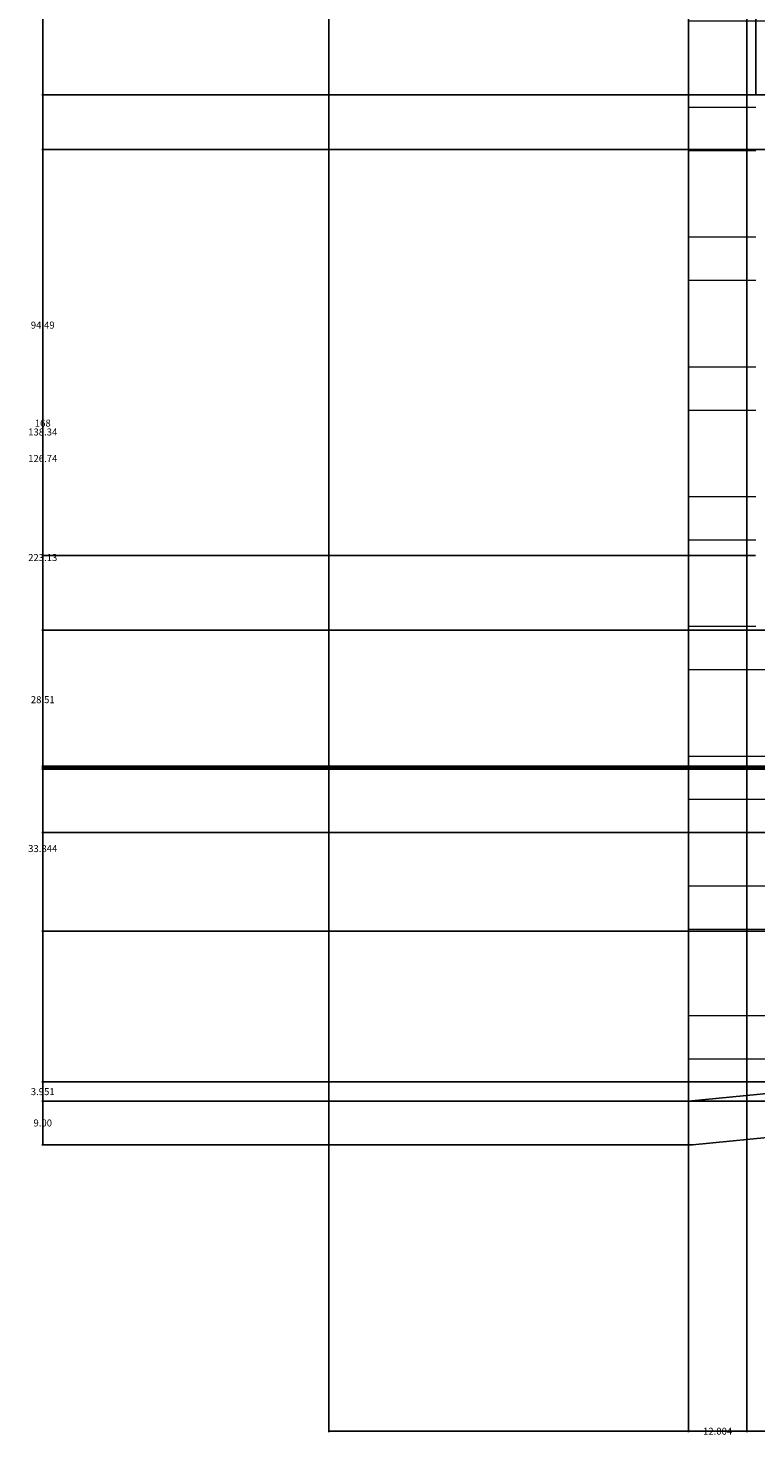
# Model space of a CAD drawing. Units: inches. Extents: x 241 to 943, y 109 to 1396.
# Tile 1 of 34: x 241 to 391, y 109 to 398. Entities that reach past the tile are written whole.
import ezdxf

# ---------------------------------------------------------------- set-up
doc = ezdxf.new("R2010")
doc.units = ezdxf.units.IN
doc.header["$MEASUREMENT"] = 0
for name, color, linetype, lineweight in [('A-ANNO-DIMS', 2, 'Continuous', 18), ('A-ELEV', 7, 'Continuous', 25), ('A-WALL-PATT', 8, 'Continuous', 13)]:
    doc.layers.add(name, color=color, linetype=linetype, lineweight=lineweight)
doc.styles.get("Standard").update_dxf_attribs({"font": 'arial.ttf'})
doc.dimstyles.get("Standard").update_dxf_attribs({"dimtxt": 1.4375, "dimasz": 0.18, "dimexe": 0.18, "dimexo": 0.0625, "dimgap": 0.09, "dimtad": 0, "dimtih": 1, "dimtoh": 1, "dimdec": 4, "dimzin": 0, "dimdsep": 46, "dimlunit": 4, "dimtxsty": 'Standard', "dimcen": 0.09, "dimadec": 0, "dimazin": 0, "dimtfac": 1, "dimtdec": 4, "dimtofl": 0, "dimtmove": 0, "dimatfit": 3, "dimfxl": 1, "dimtolj": 1, "dimtzin": 0, "dimarcsym": 0})

# ---------------------------------------------------------------- blocks, each defined once
blk = doc.blocks.new('*D4')
at = {"layer": 'A-ANNO-DIMS', "color": 0, "lineweight": -2, "transparency": 16777216}
for p, q in [((820.84, 232.77), (820.84, 109.81)), ((377.04, 177.64), (377.04, 109.81)), ((377.22, 109.99), (596.39, 109.99)), ((820.66, 109.99), (601.48, 109.99))]:
    blk.add_line(p, q, dxfattribs=at)
at = {"layer": 'A-ANNO-DIMS', "color": 0, "transparency": 16777216}
for points in [[(377.22, 110.02), (377.22, 109.96), (377.04, 109.99)], [(820.66, 110.02), (820.66, 109.96), (820.84, 109.99)]]:
    blk.add_solid(points, dxfattribs=at)
at = {"layer": 'Defpoints', "color": 0, "transparency": 16777216}
for p in [(820.84, 232.83), (377.04, 177.7), (820.84, 109.99)]:
    blk.add_point(p, dxfattribs=at)
at = {"layer": 'A-ANNO-DIMS', "color": 0, "transparency": 16777216, "insert": (598.94, 109.99), "char_height": 1.438, "attachment_point": 5}
blk.add_mtext('\\A1;443.8', dxfattribs=at)
blk = doc.blocks.new('*D5')
at = {"layer": 'A-ANNO-DIMS', "color": 0, "lineweight": -2, "transparency": 16777216}
for p, q in [((303.24, 177.8), (303.24, 1395.05)), ((377.04, 177.76), (377.04, 1395.05)), ((303.42, 1394.87), (338.18, 1394.87)), ((376.86, 1394.87), (342.09, 1394.87))]:
    blk.add_line(p, q, dxfattribs=at)
at = {"layer": 'A-ANNO-DIMS', "color": 0, "transparency": 16777216}
for points in [[(303.42, 1394.9), (303.42, 1394.84), (303.24, 1394.87)], [(376.86, 1394.9), (376.86, 1394.84), (377.04, 1394.87)]]:
    blk.add_solid(points, dxfattribs=at)
at = {"layer": 'Defpoints', "color": 0, "transparency": 16777216}
for p in [(377.04, 1394.87), (303.24, 177.74), (377.04, 177.7)]:
    blk.add_point(p, dxfattribs=at)
at = {"layer": 'A-ANNO-DIMS', "color": 0, "transparency": 16777216, "insert": (340.14, 1394.87), "char_height": 1.438, "attachment_point": 5}
blk.add_mtext('\\A1;73.8', dxfattribs=at)
blk = doc.blocks.new('*D7')
at = {"layer": 'A-ANNO-DIMS', "color": 0, "lineweight": -2, "transparency": 16777216}
for p, q in [((508.24, 1336.12), (244.31, 1336.12)), ((244.49, 1335.94), (244.49, 753.25)), ((244.49, 168.92), (244.49, 751.6)), ((303.17, 168.74), (244.31, 168.74))]:
    blk.add_line(p, q, dxfattribs=at)
at = {"layer": 'A-ANNO-DIMS', "color": 0, "transparency": 16777216}
for points in [[(244.46, 1335.94), (244.52, 1335.94), (244.49, 1336.12)], [(244.46, 168.92), (244.52, 168.92), (244.49, 168.74)]]:
    blk.add_solid(points, dxfattribs=at)
at = {"layer": 'Defpoints', "color": 0, "transparency": 16777216}
for p in [(244.49, 1336.12), (508.31, 1336.12), (303.24, 168.74)]:
    blk.add_point(p, dxfattribs=at)
at = {"layer": 'A-ANNO-DIMS', "color": 0, "transparency": 16777216, "insert": (244.49, 752.43), "char_height": 1.438, "attachment_point": 5}
blk.add_mtext('\\A1;1167.4', dxfattribs=at)
blk = doc.blocks.new('*D8')
at = {"layer": 'A-ANNO-DIMS', "color": 0, "lineweight": -2, "transparency": 16777216}
for p, q in [((377.04, 396.94), (377.04, 1395.05)), ((390.89, 384.24), (390.89, 1395.05)), ((377.22, 1394.87), (380.96, 1394.87)), ((390.71, 1394.87), (386.97, 1394.87))]:
    blk.add_line(p, q, dxfattribs=at)
at = {"layer": 'A-ANNO-DIMS', "color": 0, "transparency": 16777216}
for points in [[(377.22, 1394.9), (377.22, 1394.84), (377.04, 1394.87)], [(390.71, 1394.9), (390.71, 1394.84), (390.89, 1394.87)]]:
    blk.add_solid(points, dxfattribs=at)
at = {"layer": 'Defpoints', "color": 0, "transparency": 16777216}
for p in [(390.89, 1394.87), (377.04, 396.88), (390.89, 384.18)]:
    blk.add_point(p, dxfattribs=at)
at = {"layer": 'A-ANNO-DIMS', "color": 0, "transparency": 16777216, "insert": (383.97, 1394.87), "char_height": 1.438, "attachment_point": 5}
blk.add_mtext('\\A1;13.856', dxfattribs=at)
blk = doc.blocks.new('*D9')
at = {"layer": 'A-ANNO-DIMS', "color": 0, "lineweight": -2, "transparency": 16777216}
for p, q in [((390.89, 384.24), (390.89, 1395.05)), ((462.11, 384.24), (462.11, 1395.05)), ((391.07, 1394.87), (424.13, 1394.87)), ((461.93, 1394.87), (428.87, 1394.87))]:
    blk.add_line(p, q, dxfattribs=at)
at = {"layer": 'A-ANNO-DIMS', "color": 0, "transparency": 16777216}
for points in [[(391.07, 1394.9), (391.07, 1394.84), (390.89, 1394.87)], [(461.93, 1394.9), (461.93, 1394.84), (462.11, 1394.87)]]:
    blk.add_solid(points, dxfattribs=at)
at = {"layer": 'Defpoints', "color": 0, "transparency": 16777216}
for p in [(462.11, 1394.87), (390.89, 384.18), (462.11, 384.18)]:
    blk.add_point(p, dxfattribs=at)
at = {"layer": 'A-ANNO-DIMS', "color": 0, "transparency": 16777216, "insert": (426.5, 1394.87), "char_height": 1.438, "attachment_point": 5}
blk.add_mtext('\\A1;71.21', dxfattribs=at)
blk = doc.blocks.new('*D20')
at = {"layer": 'A-ANNO-DIMS', "color": 0, "lineweight": -2, "transparency": 16777216}
for p, q in [((376.98, 400.83), (244.31, 400.83)), ((244.49, 400.65), (244.49, 290.09)), ((244.49, 177.88), (244.49, 288.44)), ((376.98, 177.7), (244.31, 177.7))]:
    blk.add_line(p, q, dxfattribs=at)
at = {"layer": 'A-ANNO-DIMS', "color": 0, "transparency": 16777216}
for points in [[(244.46, 400.65), (244.52, 400.65), (244.49, 400.83)], [(244.46, 177.88), (244.52, 177.88), (244.49, 177.7)]]:
    blk.add_solid(points, dxfattribs=at)
at = {"layer": 'Defpoints', "color": 0, "transparency": 16777216}
for p in [(244.49, 400.83), (377.04, 400.83), (377.04, 177.7)]:
    blk.add_point(p, dxfattribs=at)
at = {"layer": 'A-ANNO-DIMS', "color": 0, "transparency": 16777216, "insert": (244.49, 289.26), "char_height": 1.438, "attachment_point": 5}
blk.add_mtext('\\A1;223.13', dxfattribs=at)
blk = doc.blocks.new('*D30')
at = {"layer": 'A-ANNO-DIMS', "color": 0, "lineweight": -2, "transparency": 16777216}
for p, q in [((390.83, 384.18), (244.31, 384.18)), ((244.49, 384), (244.49, 337.76)), ((244.49, 289.87), (244.49, 336.11)), ((390.83, 289.69), (244.31, 289.69))]:
    blk.add_line(p, q, dxfattribs=at)
at = {"layer": 'A-ANNO-DIMS', "color": 0, "transparency": 16777216}
for points in [[(244.46, 384), (244.52, 384), (244.49, 384.18)], [(244.46, 289.87), (244.52, 289.87), (244.49, 289.69)]]:
    blk.add_solid(points, dxfattribs=at)
at = {"layer": 'Defpoints', "color": 0, "transparency": 16777216}
for p in [(244.49, 384.18), (390.89, 384.18), (390.89, 289.69)]:
    blk.add_point(p, dxfattribs=at)
at = {"layer": 'A-ANNO-DIMS', "color": 0, "transparency": 16777216, "insert": (244.49, 336.94), "char_height": 1.438, "attachment_point": 5}
blk.add_mtext('\\A1;94.49', dxfattribs=at)
blk = doc.blocks.new('*D41')
at = {"layer": 'A-ANNO-DIMS', "color": 0, "lineweight": -2, "transparency": 16777216}
for p, q in [((820.77, 400.83), (244.31, 400.83)), ((244.49, 400.65), (244.49, 317.65)), ((244.49, 233.01), (244.49, 316.01)), ((820.77, 232.83), (244.31, 232.83))]:
    blk.add_line(p, q, dxfattribs=at)
at = {"layer": 'A-ANNO-DIMS', "color": 0, "transparency": 16777216}
for points in [[(244.46, 400.65), (244.52, 400.65), (244.49, 400.83)], [(244.46, 233.01), (244.52, 233.01), (244.49, 232.83)]]:
    blk.add_solid(points, dxfattribs=at)
at = {"layer": 'Defpoints', "color": 0, "transparency": 16777216}
for p in [(244.49, 400.83), (820.84, 400.83), (820.84, 232.83)]:
    blk.add_point(p, dxfattribs=at)
at = {"layer": 'A-ANNO-DIMS', "color": 0, "transparency": 16777216, "insert": (244.49, 316.83), "char_height": 1.438, "attachment_point": 5}
blk.add_mtext('\\A1;168', dxfattribs=at)
blk = doc.blocks.new('*D50')
at = {"layer": 'A-ANNO-DIMS', "color": 0, "lineweight": -2, "transparency": 16777216}
for p, q in [((651.55, 246.46), (244.31, 246.46)), ((244.49, 246.28), (244.49, 230.36)), ((244.49, 212.79), (244.49, 228.71)), ((651.72, 212.61), (244.31, 212.61))]:
    blk.add_line(p, q, dxfattribs=at)
at = {"layer": 'A-ANNO-DIMS', "color": 0, "transparency": 16777216}
for points in [[(244.46, 246.28), (244.52, 246.28), (244.49, 246.46)], [(244.46, 212.79), (244.52, 212.79), (244.49, 212.61)]]:
    blk.add_solid(points, dxfattribs=at)
at = {"layer": 'Defpoints', "color": 0, "transparency": 16777216}
for p in [(244.49, 246.46), (651.61, 246.46), (651.79, 212.61)]:
    blk.add_point(p, dxfattribs=at)
at = {"layer": 'A-ANNO-DIMS', "color": 0, "transparency": 16777216, "insert": (244.49, 229.54), "char_height": 1.438, "attachment_point": 5}
blk.add_mtext('\\A1;33.844', dxfattribs=at)
blk = doc.blocks.new('*D51')
at = {"layer": 'A-ANNO-DIMS', "color": 0, "lineweight": -2, "transparency": 16777216}
for p, q in [((595.25, 372.94), (244.31, 372.94)), ((244.49, 372.76), (244.49, 310.39)), ((244.49, 246.38), (244.49, 308.74)), ((595.25, 246.2), (244.31, 246.2))]:
    blk.add_line(p, q, dxfattribs=at)
at = {"layer": 'A-ANNO-DIMS', "color": 0, "transparency": 16777216}
for points in [[(244.46, 372.76), (244.52, 372.76), (244.49, 372.94)], [(244.46, 246.38), (244.52, 246.38), (244.49, 246.2)]]:
    blk.add_solid(points, dxfattribs=at)
at = {"layer": 'Defpoints', "color": 0, "transparency": 16777216}
for p in [(244.49, 372.94), (595.31, 372.94), (595.31, 246.2)]:
    blk.add_point(p, dxfattribs=at)
at = {"layer": 'A-ANNO-DIMS', "color": 0, "transparency": 16777216, "insert": (244.49, 309.57), "char_height": 1.438, "attachment_point": 5}
blk.add_mtext('\\A1;126.74', dxfattribs=at)
blk = doc.blocks.new('*D52')
at = {"layer": 'A-ANNO-DIMS', "color": 0, "lineweight": -2, "transparency": 16777216}
for p, q in [((530.17, 384.18), (244.31, 384.18)), ((244.49, 384), (244.49, 315.83)), ((244.49, 246.02), (244.49, 314.18)), ((530.17, 245.84), (244.31, 245.84))]:
    blk.add_line(p, q, dxfattribs=at)
at = {"layer": 'A-ANNO-DIMS', "color": 0, "transparency": 16777216}
for points in [[(244.46, 384), (244.52, 384), (244.49, 384.18)], [(244.46, 246.02), (244.52, 246.02), (244.49, 245.84)]]:
    blk.add_solid(points, dxfattribs=at)
at = {"layer": 'Defpoints', "color": 0, "transparency": 16777216}
for p in [(244.49, 384.18), (530.23, 384.18), (530.23, 245.84)]:
    blk.add_point(p, dxfattribs=at)
at = {"layer": 'A-ANNO-DIMS', "color": 0, "transparency": 16777216, "insert": (244.49, 315.01), "char_height": 1.438, "attachment_point": 5}
blk.add_mtext('\\A1;138.34', dxfattribs=at)
blk = doc.blocks.new('*D73')
at = {"layer": 'A-ANNO-DIMS', "color": 0, "lineweight": -2, "transparency": 16777216}
for p, q in [((303.17, 177.74), (244.31, 177.74)), ((244.49, 177.56), (244.49, 174.06)), ((244.49, 168.92), (244.49, 172.42)), ((303.17, 168.74), (244.31, 168.74))]:
    blk.add_line(p, q, dxfattribs=at)
at = {"layer": 'A-ANNO-DIMS', "color": 0, "transparency": 16777216}
for points in [[(244.46, 177.56), (244.52, 177.56), (244.49, 177.74)], [(244.46, 168.92), (244.52, 168.92), (244.49, 168.74)]]:
    blk.add_solid(points, dxfattribs=at)
at = {"layer": 'Defpoints', "color": 0, "transparency": 16777216}
for p in [(244.49, 177.74), (303.24, 177.74), (303.24, 168.74)]:
    blk.add_point(p, dxfattribs=at)
at = {"layer": 'A-ANNO-DIMS', "color": 0, "transparency": 16777216, "insert": (244.49, 173.24), "char_height": 1.438, "attachment_point": 5}
blk.add_mtext('\\A1;9.00', dxfattribs=at)
blk = doc.blocks.new('*D74')
at = {"layer": 'A-ANNO-DIMS', "color": 0, "lineweight": -2, "transparency": 16777216}
for p, q in [((417.09, 181.59), (417.09, 109.81)), ((377.04, 177.64), (377.04, 109.81)), ((377.22, 109.99), (394.52, 109.99)), ((416.91, 109.99), (399.61, 109.99))]:
    blk.add_line(p, q, dxfattribs=at)
at = {"layer": 'A-ANNO-DIMS', "color": 0, "transparency": 16777216}
for points in [[(377.22, 110.02), (377.22, 109.96), (377.04, 109.99)], [(416.91, 110.02), (416.91, 109.96), (417.09, 109.99)]]:
    blk.add_solid(points, dxfattribs=at)
at = {"layer": 'Defpoints', "color": 0, "transparency": 16777216}
for p in [(417.09, 181.65), (377.04, 177.7), (417.09, 109.99)]:
    blk.add_point(p, dxfattribs=at)
at = {"layer": 'A-ANNO-DIMS', "color": 0, "transparency": 16777216, "insert": (397.07, 109.99), "char_height": 1.438, "attachment_point": 5}
blk.add_mtext('\\A1;40.05', dxfattribs=at)
blk = doc.blocks.new('*D75')
at = {"layer": 'A-ANNO-DIMS', "color": 0, "lineweight": -2, "transparency": 16777216}
for p, q in [((667.46, 214.52), (940.6, 214.52)), ((940.42, 214.34), (940.42, 196.93)), ((940.42, 177.88), (940.42, 195.28)), ((377.1, 177.7), (940.6, 177.7))]:
    blk.add_line(p, q, dxfattribs=at)
at = {"layer": 'A-ANNO-DIMS', "color": 0, "transparency": 16777216}
for points in [[(940.39, 214.34), (940.45, 214.34), (940.42, 214.52)], [(940.39, 177.88), (940.45, 177.88), (940.42, 177.7)]]:
    blk.add_solid(points, dxfattribs=at)
at = {"layer": 'Defpoints', "color": 0, "transparency": 16777216}
for p in [(667.39, 214.52), (940.42, 214.52), (377.04, 177.7)]:
    blk.add_point(p, dxfattribs=at)
at = {"layer": 'A-ANNO-DIMS', "color": 0, "transparency": 16777216, "insert": (940.42, 196.11), "char_height": 1.438, "attachment_point": 5}
blk.add_mtext('\\A1;36.82', dxfattribs=at)
blk = doc.blocks.new('*D81')
at = {"layer": 'A-ANNO-DIMS', "color": 0, "lineweight": -2, "transparency": 16777216}
for p, q in [((462.04, 274.35), (244.31, 274.35)), ((244.49, 274.17), (244.49, 260.92)), ((244.49, 246.02), (244.49, 259.27)), ((530.17, 245.84), (244.31, 245.84))]:
    blk.add_line(p, q, dxfattribs=at)
at = {"layer": 'A-ANNO-DIMS', "color": 0, "transparency": 16777216}
for points in [[(244.46, 274.17), (244.52, 274.17), (244.49, 274.35)], [(244.46, 246.02), (244.52, 246.02), (244.49, 245.84)]]:
    blk.add_solid(points, dxfattribs=at)
at = {"layer": 'Defpoints', "color": 0, "transparency": 16777216}
for p in [(244.49, 274.35), (462.11, 274.35), (530.23, 245.84)]:
    blk.add_point(p, dxfattribs=at)
at = {"layer": 'A-ANNO-DIMS', "color": 0, "transparency": 16777216, "insert": (244.49, 260.09), "char_height": 1.438, "attachment_point": 5}
blk.add_mtext('\\A1;28.51', dxfattribs=at)
blk = doc.blocks.new('*D91')
at = {"layer": 'A-ANNO-DIMS', "color": 0, "lineweight": -2, "transparency": 16777216}
for p, q in [((377.04, 1070.79), (377.04, 109.81)), ((389.04, 1070.79), (389.04, 109.81)), ((377.22, 109.99), (380.04, 109.99)), ((388.86, 109.99), (386.04, 109.99))]:
    blk.add_line(p, q, dxfattribs=at)
at = {"layer": 'A-ANNO-DIMS', "color": 0, "transparency": 16777216}
for points in [[(377.22, 110.02), (377.22, 109.96), (377.04, 109.99)], [(388.86, 110.02), (388.86, 109.96), (389.04, 109.99)]]:
    blk.add_solid(points, dxfattribs=at)
at = {"layer": 'Defpoints', "color": 0, "transparency": 16777216}
for p in [(377.04, 1070.85), (389.04, 1070.85), (389.04, 109.99)]:
    blk.add_point(p, dxfattribs=at)
at = {"layer": 'A-ANNO-DIMS', "color": 0, "transparency": 16777216, "insert": (383.04, 109.99), "char_height": 1.438, "attachment_point": 5}
blk.add_mtext('\\A1;12.004', dxfattribs=at)
blk = doc.blocks.new('*D97')
at = {"layer": 'A-ANNO-DIMS', "color": 0, "lineweight": -2, "transparency": 16777216}
for p, q in [((881.67, 223.77), (881.67, 109.81)), ((303.24, 168.68), (303.24, 109.81)), ((303.42, 109.99), (589.38, 109.99)), ((881.49, 109.99), (595.53, 109.99))]:
    blk.add_line(p, q, dxfattribs=at)
at = {"layer": 'A-ANNO-DIMS', "color": 0, "transparency": 16777216}
for points in [[(303.42, 110.02), (303.42, 109.96), (303.24, 109.99)], [(881.49, 110.02), (881.49, 109.96), (881.67, 109.99)]]:
    blk.add_solid(points, dxfattribs=at)
at = {"layer": 'Defpoints', "color": 0, "transparency": 16777216}
for p in [(881.67, 223.83), (303.24, 168.74), (881.67, 109.99)]:
    blk.add_point(p, dxfattribs=at)
at = {"layer": 'A-ANNO-DIMS', "color": 0, "transparency": 16777216, "insert": (592.45, 109.99), "char_height": 1.438, "attachment_point": 5}
blk.add_mtext('\\A1;578.43', dxfattribs=at)
blk = doc.blocks.new('*D98')
at = {"layer": 'A-ANNO-DIMS', "color": 0, "lineweight": -2, "transparency": 16777216}
for p, q in [((417.03, 181.65), (244.31, 181.65)), ((244.49, 181.47), (244.49, 180.5)), ((376.98, 177.7), (244.31, 177.7)), ((244.49, 177.88), (244.49, 178.85))]:
    blk.add_line(p, q, dxfattribs=at)
at = {"layer": 'A-ANNO-DIMS', "color": 0, "transparency": 16777216}
for points in [[(244.46, 181.47), (244.52, 181.47), (244.49, 181.65)], [(244.46, 177.88), (244.52, 177.88), (244.49, 177.7)]]:
    blk.add_solid(points, dxfattribs=at)
at = {"layer": 'Defpoints', "color": 0, "transparency": 16777216}
for p in [(244.49, 181.65), (417.09, 181.65), (377.04, 177.7)]:
    blk.add_point(p, dxfattribs=at)
at = {"layer": 'A-ANNO-DIMS', "color": 0, "transparency": 16777216, "insert": (244.49, 179.67), "char_height": 1.438, "attachment_point": 5}
blk.add_mtext('\\A1;3.951', dxfattribs=at)
blk = doc.blocks.new('*D147')
at = {"layer": 'A-ANNO-DIMS', "color": 0, "lineweight": -2, "transparency": 16777216}
for p, q in [((389.04, 734.79), (389.04, 109.81)), ((413.12, 734.79), (413.12, 109.81)), ((389.22, 109.99), (398, 109.99)), ((412.94, 109.99), (404.17, 109.99))]:
    blk.add_line(p, q, dxfattribs=at)
at = {"layer": 'A-ANNO-DIMS', "color": 0, "transparency": 16777216}
for points in [[(389.22, 110.02), (389.22, 109.96), (389.04, 109.99)], [(412.94, 110.02), (412.94, 109.96), (413.12, 109.99)]]:
    blk.add_solid(points, dxfattribs=at)
at = {"layer": 'Defpoints', "color": 0, "transparency": 16777216}
for p in [(389.04, 734.85), (413.12, 734.85), (413.12, 109.99)]:
    blk.add_point(p, dxfattribs=at)
at = {"layer": 'A-ANNO-DIMS', "color": 0, "transparency": 16777216, "insert": (401.08, 109.99), "char_height": 1.438, "attachment_point": 5}
blk.add_mtext('\\A1;24.076', dxfattribs=at)

msp = doc.modelspace()

# ---------------------------------------------------------------- hatches: boundary and pattern name
at = {"layer": 'A-WALL-PATT'}
h = msp.add_hatch(dxfattribs=at)
h.set_pattern_fill('ANSI32', color=256, scale=71, angle=135)
h.paths.add_polyline_path([(820.8374, 568.8295), (792.691, 568.8295), (792.691, 496.4395), (651.5974, 496.4395), (651.5974, 568.8295), (617.7594, 568.8295), (618.9643, 400.8295), (417.0913, 400.8295), (377.0391, 400.8295), (377.0391, 398.8538), (377.0391, 396.8782), (377.0391, 228.8782), (377.0391, 177.6977), (416.5078, 181.5724), (417.0913, 181.649), (530.2303, 196.5065), (530.2303, 384.1784), (650.907, 384.1784), (651.7861, 212.4693), (667.3935, 214.5189), (667.3935, 289.9984), (794.0275, 289.9984), (794.0275, 232.8295), (820.8374, 232.8295), (820.8374, 400.8295)])
h.paths.add_polyline_path([(500.3323, 384.1784), (500.3323, 289.6933), (500.3323, 274.3507), (479.596, 274.3507), (479.596, 289.6933), (479.596, 384.1784)], flags=16)
h.paths.add_polyline_path([(498.3323, 382.1784), (498.3323, 291.6933), (481.596, 291.6933), (481.596, 382.1784)], flags=0)
h.paths.add_polyline_path([(462.1074, 384.1784), (462.1074, 289.6933), (462.1074, 277.4626), (462.1074, 274.3507), (390.895, 274.3507), (390.895, 277.4626), (390.895, 289.6933), (390.895, 384.1784)], flags=16)
h.paths.add_polyline_path([(460.1074, 382.1784), (460.1074, 291.6933), (392.895, 291.6933), (392.895, 382.1784)], flags=0)
h.paths.add_polyline_path([(595.3136, 372.9401), (641.6196, 372.9401), (641.6196, 246.4081), (651.6121, 246.4593), (650.907, 384.1784), (530.2303, 384.1784), (530.2303, 245.8378), (595.3136, 246.1711)], flags=17)

# ---------------------------------------------------------------- linework, layer by layer
at = {"layer": 'A-ELEV'}
for p, q in [((377.0391, 396.8782), (377.0391, 400.8295)), ((377.0391, 228.8782), (377.0391, 396.8782)), ((377.0391, 177.6977), (377.0391, 228.8782)), ((416.5078, 181.5724), (377.0391, 177.6977)), ((377.0391, 177.6977), (303.2358, 177.7407)), ((303.2358, 168.7407), (303.2358, 177.7407)), ((417.0913, 172.649), (377.9184, 168.7407)), ((377.9184, 168.7407), (303.2358, 168.7407))]:
    msp.add_line(p, q, dxfattribs=at)

# ---------------------------------------------------------------- dimensions: what is measured, and where the dimension line sits
at = {"layer": 'A-ANNO-DIMS'}
for base, p1, p2, override, picture, middle in [((377.0391, 1394.8654), (303.2358, 177.7407), (377.0391, 177.6977), {"dimdec": 1, "dimlfac": 1, "dimrnd": 0, "dimzin": 0, "dimdsep": 46, "dimlunit": 2}, '*D5', (340.1375, 1394.8654)), ((390.895, 1394.8654), (377.0391, 396.8782), (390.895, 384.1784), {"dimdec": 3, "dimlfac": 1, "dimrnd": 0, "dimzin": 0, "dimdsep": 46, "dimlunit": 2}, '*D8', (383.9671, 1394.8654)), ((462.1074, 1394.8654), (390.895, 384.1784), (462.1074, 384.1784), {"dimdec": 2, "dimlfac": 1, "dimrnd": 0, "dimzin": 0, "dimdsep": 46, "dimlunit": 2}, '*D9', (426.5012, 1394.8654)), ((389.0429, 109.9907), (377.0391, 1070.8538), (389.0429, 1070.8538), {"dimdec": 3, "dimlfac": 1, "dimrnd": 0, "dimzin": 0, "dimdsep": 46, "dimlunit": 2}, '*D91', (383.041, 109.9907)), ((413.1187, 109.9907), (389.0429, 734.8538), (413.1187, 734.8538), {"dimdec": 3, "dimlfac": 1, "dimrnd": 0, "dimzin": 0, "dimdsep": 46, "dimlunit": 2}, '*D147', (401.0808, 109.9907)), ((820.8374, 109.9907), (377.0391, 177.6977), (820.8374, 232.8295), {"dimdec": 1, "dimlfac": 1, "dimrnd": 0, "dimzin": 0, "dimdsep": 46, "dimlunit": 2}, '*D4', (598.9383, 109.9907)), ((881.667, 109.9907), (303.2358, 168.7407), (881.667, 223.8295), {"dimdec": 2, "dimlfac": 1, "dimrnd": 0, "dimzin": 0, "dimdsep": 46, "dimlunit": 2}, '*D97', (592.4514, 109.9907)), ((417.0913, 109.9907), (377.0391, 177.6977), (417.0913, 181.649), {"dimdec": 2, "dimlfac": 1, "dimrnd": 0, "dimzin": 0, "dimdsep": 46, "dimlunit": 2}, '*D74', (397.0652, 109.9907))]:
    dim = msp.add_linear_dim(base=base, p1=p1, p2=p2, dimstyle='Standard', override=override, dxfattribs=at)
    dim.commit()
    dim.dimension.update_dxf_attribs({"geometry": picture, "text_midpoint": middle})
for base, p1, p2, override, picture, middle in [((244.4858, 1336.1154), (303.2358, 168.7407), (508.3064, 1336.1154), {"dimdec": 1, "dimlfac": 1, "dimrnd": 0, "dimzin": 0, "dimdsep": 46, "dimlunit": 2}, '*D7', (244.4858, 752.4281)), ((244.4858, 400.8295), (377.0391, 177.6977), (377.0391, 400.8295), {"dimdec": 2, "dimlfac": 1, "dimrnd": 0, "dimzin": 0, "dimdsep": 46, "dimlunit": 2}, '*D20', (244.4858, 289.2636)), ((244.4858, 400.8295), (820.8374, 232.8295), (820.8374, 400.8295), {"dimdec": 0, "dimlfac": 1, "dimrnd": 0, "dimzin": 0, "dimdsep": 46, "dimlunit": 2}, '*D41', (244.4858, 316.8295)), ((244.4858, 384.1784), (530.2303, 245.8378), (530.2303, 384.1784), {"dimdec": 2, "dimlfac": 1, "dimrnd": 0, "dimzin": 0, "dimdsep": 46, "dimlunit": 2}, '*D52', (244.4858, 315.0081)), ((244.4858, 384.1784), (390.895, 289.6933), (390.895, 384.1784), {"dimdec": 2, "dimlfac": 1, "dimrnd": 0, "dimzin": 0, "dimdsep": 46, "dimlunit": 2}, '*D30', (244.4858, 336.9358)), ((244.4858, 372.9401), (595.3136, 246.1966), (595.3136, 372.9401), {"dimdec": 2, "dimlfac": 1, "dimrnd": 0, "dimzin": 0, "dimdsep": 46, "dimlunit": 2}, '*D51', (244.4858, 309.5684)), ((244.4858, 274.3507), (530.2303, 245.8378), (462.1074, 274.3507), {"dimdec": 2, "dimlfac": 1, "dimrnd": 0, "dimzin": 0, "dimdsep": 46, "dimlunit": 2}, '*D81', (244.4858, 260.0943)), ((244.4858, 246.4593), (651.7854, 212.6149), (651.6121, 246.4593), {"dimdec": 3, "dimlfac": 1, "dimrnd": 0, "dimzin": 0, "dimdsep": 46, "dimlunit": 2}, '*D50', (244.4858, 229.5371)), ((940.417, 214.5189), (377.0391, 177.6977), (667.3935, 214.5189), {"dimdec": 2, "dimlfac": 1, "dimrnd": 0, "dimzin": 0, "dimdsep": 46, "dimlunit": 2}, '*D75', (940.417, 196.1083)), ((244.4858, 181.649), (377.0391, 177.6977), (417.0913, 181.649), {"dimdec": 3, "dimlfac": 1, "dimrnd": 0, "dimzin": 0, "dimdsep": 46, "dimlunit": 2}, '*D98', (244.4858, 179.6733)), ((244.4858, 177.7407), (303.2358, 168.7407), (303.2358, 177.7407), {"dimdec": 2, "dimlfac": 1, "dimrnd": 0, "dimzin": 0, "dimdsep": 46, "dimlunit": 2}, '*D73', (244.4858, 173.2407))]:
    dim = msp.add_linear_dim(base=base, p1=p1, p2=p2, angle=90, dimstyle='Standard', override=override, dxfattribs=at)
    dim.commit()
    dim.dimension.update_dxf_attribs({"geometry": picture, "text_midpoint": middle})

doc.saveas('drawing.dxf')
